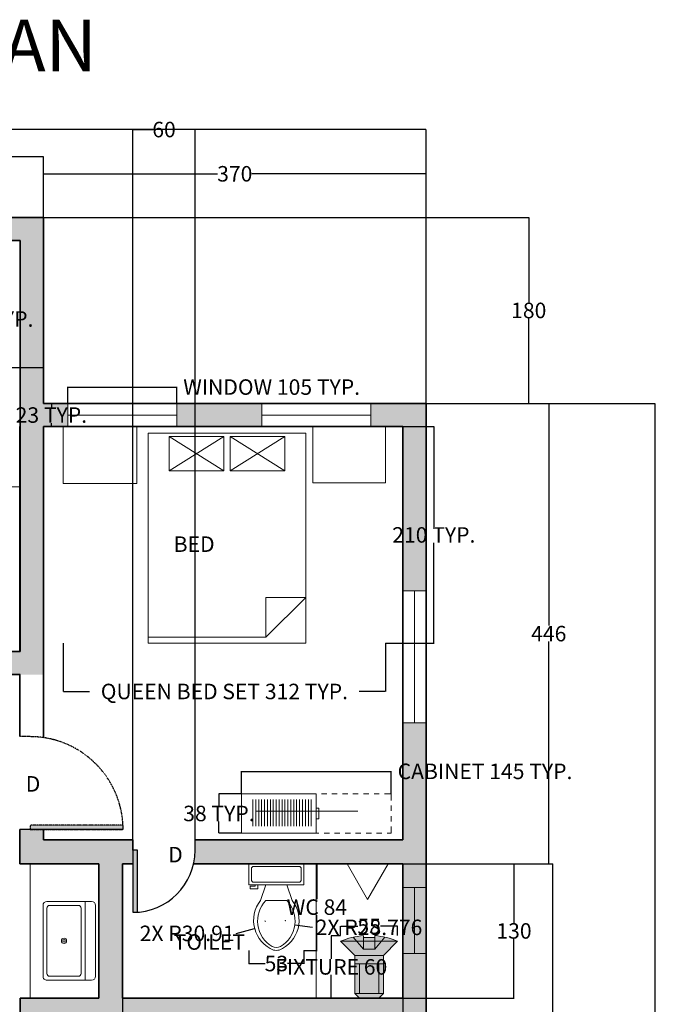
# Model space of a CAD drawing. Units: centimetres. Extents: x 355 to 1615, y 1030 to 2729.
# Tile 3 of 3: x 978 to 1615, y 1776 to 2729. Entities that reach past the tile are written whole.
import ezdxf

# ---------------------------------------------------------------- set-up
doc = ezdxf.new("R2010")
doc.units = ezdxf.units.CM
doc.header["$MEASUREMENT"] = 0
doc.linetypes.add('HIDDEN', pattern=[0.375, 0.25, -0.125])
for name, color, linetype, lineweight in [('A-ANNO-DIMS', 2, 'Continuous', 18), ('A-ANNO-TEXT', 7, 'Continuous', 25), ('A-AREA-IDEN', 7, 'Continuous', 25), ('A-DOOR', 4, 'Continuous', 25), ('A-DOOR-HIDN', 4, 'HIDDEN', 25), ('A-FLOR-CASE', 9, 'Continuous', 20), ('A-FLOR-FIXT', 9, 'Continuous', 18), ('A-FURN', 8, 'Continuous', 18), ('A-GLAZ', 4, 'Continuous', 18), ('A-WALL', 7, 'Continuous', 35), ('A-WALL-PATT', 5, 'Continuous', 13)]:
    doc.layers.add(name, color=color, linetype=linetype, lineweight=lineweight)
doc.styles.get("Standard").update_dxf_attribs({"font": 'arial.ttf'})
doc.dimstyles.get("Standard").update_dxf_attribs({"dimtxt": 15, "dimasz": 0.18, "dimexe": 0.18, "dimexo": 0.0625, "dimgap": 0.09, "dimtad": 0, "dimtih": 1, "dimtoh": 1, "dimdec": 0, "dimzin": 0, "dimdsep": 46, "dimtxsty": 'Standard', "dimcen": 0.09, "dimadec": 0, "dimazin": 0, "dimtfac": 1, "dimtdec": 0, "dimtofl": 0, "dimtmove": 0, "dimatfit": 3, "dimfxl": 1, "dimtolj": 1, "dimtzin": 0, "dimarcsym": 0})

# ---------------------------------------------------------------- blocks, each defined once
blk = doc.blocks.new('*D8')
at = {"layer": 'A-ANNO-DIMS', "color": 0, "lineweight": -2, "transparency": 16777216}
for p, q in [((611.23, 2537.61), (611.23, 2391.81)), ((1001.23, 2537.61), (1001.23, 2391.81)), ((611.41, 2391.99), (789.6, 2391.99)), ((1001.05, 2391.99), (822.86, 2391.99))]:
    blk.add_line(p, q, dxfattribs=at)
at = {"layer": 'A-ANNO-DIMS', "color": 0, "transparency": 16777216}
for points in [[(611.41, 2392.02), (611.41, 2391.96), (611.23, 2391.99)], [(1001.05, 2392.02), (1001.05, 2391.96), (1001.23, 2391.99)]]:
    blk.add_solid(points, dxfattribs=at)
at = {"layer": 'Defpoints', "color": 0, "transparency": 16777216}
for p in [(611.23, 2537.67), (1001.23, 2537.67), (1001.23, 2391.99)]:
    blk.add_point(p, dxfattribs=at)
at = {"layer": 'A-ANNO-DIMS', "color": 0, "transparency": 16777216, "insert": (806.23, 2391.99), "char_height": 15, "attachment_point": 5}
blk.add_mtext('\\A1;390', dxfattribs=at)
blk = doc.blocks.new('*U3')
for p, q in [((0, 0), (0, -100)), ((-900, 0), (-900, -100))]:
    blk.add_line(p, q)
blk.add_lwpolyline([(0, 0), (0, 900), (-43.75, 900), (-43.75, 0)], close=True)
blk.add_arc((0, 0), 900, 90, 180)
blk = doc.blocks.new('*U14')
for p, q in [((0, 0), (0, 100)), ((600, 0), (600, 100))]:
    blk.add_line(p, q)
blk.add_lwpolyline([(0, 0), (0, -600), (43.75, -600), (43.75, 0)], close=True)
blk.add_arc((0, 0), 600, 270, 0)
blk = doc.blocks.new('Toilet - top')
for p, q in [((9.5, -6), (9.5, -2)), ((-10, -8.5), (-8, -8.5)), ((-10, -9.5), (-10, -8.5)), ((-7, -9.5), (-10, -9.5)), ((-8, -8.5), (-8, -8)), ((-7, -8), (-7, -9.5)), ((-4, -8), (-6, -14)), ((4, -8), (6, -14)), ((4, -14), (-4, -14))]:
    blk.add_line(p, q)
blk.add_lwpolyline([(10.5, -8), (10.5, 0), (-10.5, 0), (-10.5, -8)], close=True)
for points in [[(-9.5, -2), (-9.5, -6)], [(8.5, -1), (-8.5, -1)], [(-8.5, -7), (8.5, -7)]]:
    blk.add_lwpolyline(points)
for centre, radius, start, end in [((-8.62, -1.88), 0.884, 81.8699, 188.1301), ((8.62, -1.88), 0.884, 351.8699, 98.1301), ((-8.62, -6.12), 0.884, 171.8699, 278.1301), ((8.62, -6.12), 0.884, 261.8699, 8.1301), ((3.52, -21.58), 12.17, 141.4691, 247.9714), ((4.2, -21.82), 11.33, 136.3677, 238.9468), ((-3.52, -21.58), 12.17, 292.0284, 38.5307), ((-4.2, -21.82), 11.33, 301.053, 43.6321), ((0, -27.88), 4, 245.7318, 294.2682), ((0, -29), 4, 254.8605, 285.1395)]:
    blk.add_arc(centre, radius, start, end)
blk = doc.blocks.new('Sink-single - 30 in top')
blk.add_line((-15, -3.999996), (15, -3.999996))
for points in [[(-13.5, 0), (13.5, 0)], [(-15, -18.499996), (-15, -1.5)], [(15, -1.5), (15, -18.499996)], [(-13.5, -17.499996), (-13.5, -6.499996)], [(-12.5, -5.499996), (12.5, -5.499996)], [(13.5, -6.499996), (13.5, -17.499996)], [(12.5, -18.499996), (-12.5, -18.499996)], [(13.5, -19.999996), (-13.5, -19.999996)]]:
    blk.add_lwpolyline(points)
for radius in [1, 0.5]:
    blk.add_circle((0, -11.999996), radius)
for centre, radius, start, end in [((-13.5, -1.5), 1.5, 90, 180), ((13.5, -1.5), 1.5, 0, 90), ((-12.5, -6.499996), 1, 90, 180), ((12.5, -6.499996), 1, 0, 90), ((-13.5, -18.499996), 1.5, 180, 270), ((-12.5, -17.499996), 1, 180, 270), ((12.5, -17.499996), 1, 270, 0), ((13.5, -18.499996), 1.5, 270, 0)]:
    blk.add_arc(centre, radius, start, end)
blk = doc.blocks.new('Cross Pt Oval Head Screw - 10 x 20 mm side')
at = {"color": 0}
for p, q in [((0.69, 12.04), (0.69, -7.65)), ((0.69, 12.04), (5.61, 7.12)), ((3.5, 4.16), (-0.69, 7.65)), ((18.75, 7.12), (5.61, 7.12)), ((5.61, 7.12), (5.61, -2.73)), ((8.56, -2.73), (8.56, 7.12)), ((18.75, -2.73), (18.75, 7.12)), ((20.38, 5.49), (18.75, 7.12)), ((-1.2, 4.16), (-0.61, 4.16)), ((3.5, 4.16), (-0.69, 4.16)), ((-0.61, 4.16), (-0.61, 0.23)), ((3.5, 4.16), (3.5, 0.23)), ((18.75, 5.49), (8.56, 5.49)), ((20.38, -1.1), (20.38, 5.49)), ((-1.2, 0.23), (-0.61, 0.23)), ((3.5, 0.23), (-0.69, 0.23)), ((3.5, 0.23), (-0.69, -3.26)), ((0.69, -7.65), (5.61, -2.73)), ((18.75, -2.73), (5.61, -2.73)), ((18.75, -1.1), (8.56, -1.1)), ((20.38, -1.1), (18.75, -2.73))]:
    blk.add_line(p, q, dxfattribs=at)
for start, end in [(157.3801, 175.5883), (184.4117, 202.6199)]:
    blk.add_arc((24.31, 2.19), 25.59, start, end, dxfattribs=at)
blk = doc.blocks.new('*D24')
at = {"layer": 'A-ANNO-DIMS', "color": 0, "lineweight": -2, "transparency": 16777216}
for p, q in [((611.23, 2537.73), (611.23, 2596.51)), ((611.41, 2596.33), (789.6, 2596.33)), ((1001.05, 2596.33), (822.86, 2596.33)), ((1001.23, 2537.73), (1001.23, 2596.51))]:
    blk.add_line(p, q, dxfattribs=at)
at = {"layer": 'A-ANNO-DIMS', "color": 0, "transparency": 16777216}
for points in [[(611.41, 2596.36), (611.41, 2596.3), (611.23, 2596.33)], [(1001.05, 2596.36), (1001.05, 2596.3), (1001.23, 2596.33)]]:
    blk.add_solid(points, dxfattribs=at)
at = {"layer": 'Defpoints', "color": 0, "transparency": 16777216}
for p in [(1001.23, 2596.33), (611.23, 2537.67), (1001.23, 2537.67)]:
    blk.add_point(p, dxfattribs=at)
at = {"layer": 'A-ANNO-DIMS', "color": 0, "transparency": 16777216, "insert": (806.23, 2596.33), "char_height": 15, "attachment_point": 5}
blk.add_mtext('\\A1;390', dxfattribs=at)
blk = doc.blocks.new('*D25')
at = {"layer": 'A-ANNO-DIMS', "color": 0, "lineweight": -2, "transparency": 16777216}
for p, q in [((1001.23, 2357.73), (1001.23, 2580.06)), ((1001.41, 2579.88), (1169.6, 2579.88)), ((1371.05, 2579.88), (1202.86, 2579.88)), ((1371.23, 2357.73), (1371.23, 2580.06))]:
    blk.add_line(p, q, dxfattribs=at)
at = {"layer": 'A-ANNO-DIMS', "color": 0, "transparency": 16777216}
for points in [[(1001.41, 2579.91), (1001.41, 2579.85), (1001.23, 2579.88)], [(1371.05, 2579.91), (1371.05, 2579.85), (1371.23, 2579.88)]]:
    blk.add_solid(points, dxfattribs=at)
at = {"layer": 'Defpoints', "color": 0, "transparency": 16777216}
for p in [(1371.23, 2579.88), (1001.23, 2357.67), (1371.23, 2357.67)]:
    blk.add_point(p, dxfattribs=at)
at = {"layer": 'A-ANNO-DIMS', "color": 0, "transparency": 16777216, "insert": (1186.23, 2579.88), "char_height": 15, "attachment_point": 5}
blk.add_mtext('\\A1;370', dxfattribs=at)
blk = doc.blocks.new('*D26')
at = {"layer": 'A-ANNO-DIMS', "color": 0, "lineweight": -2, "transparency": 16777216}
for p, q in [((1001.29, 2537.67), (1470.72, 2537.67)), ((1470.54, 2537.49), (1470.54, 2455.42)), ((1470.54, 2357.85), (1470.54, 2439.92)), ((1001.29, 2357.67), (1470.72, 2357.67))]:
    blk.add_line(p, q, dxfattribs=at)
at = {"layer": 'A-ANNO-DIMS', "color": 0, "transparency": 16777216}
for points in [[(1470.51, 2537.49), (1470.57, 2537.49), (1470.54, 2537.67)], [(1470.51, 2357.85), (1470.57, 2357.85), (1470.54, 2357.67)]]:
    blk.add_solid(points, dxfattribs=at)
at = {"layer": 'Defpoints', "color": 0, "transparency": 16777216}
for p in [(1001.23, 2537.67), (1001.23, 2357.67), (1470.54, 2357.67)]:
    blk.add_point(p, dxfattribs=at)
at = {"layer": 'A-ANNO-DIMS', "color": 0, "transparency": 16777216, "insert": (1470.54, 2447.67), "char_height": 15, "attachment_point": 5}
blk.add_mtext('\\A1;180', dxfattribs=at)
blk = doc.blocks.new('*D27')
at = {"layer": 'A-ANNO-DIMS', "color": 0, "lineweight": -2, "transparency": 16777216}
for p, q in [((1371.29, 2357.67), (1490.09, 2357.67)), ((1489.91, 2357.49), (1489.91, 2142.67)), ((1489.91, 1912.35), (1489.91, 2127.17)), ((1371.29, 1912.17), (1490.09, 1912.17))]:
    blk.add_line(p, q, dxfattribs=at)
at = {"layer": 'A-ANNO-DIMS', "color": 0, "transparency": 16777216}
for points in [[(1489.88, 2357.49), (1489.94, 2357.49), (1489.91, 2357.67)], [(1489.88, 1912.35), (1489.94, 1912.35), (1489.91, 1912.17)]]:
    blk.add_solid(points, dxfattribs=at)
at = {"layer": 'Defpoints', "color": 0, "transparency": 16777216}
for p in [(1371.23, 2357.67), (1371.23, 1912.17), (1489.91, 1912.17)]:
    blk.add_point(p, dxfattribs=at)
at = {"layer": 'A-ANNO-DIMS', "color": 0, "transparency": 16777216, "insert": (1489.91, 2134.92), "char_height": 15, "attachment_point": 5}
blk.add_mtext('\\A1;446', dxfattribs=at)
blk = doc.blocks.new('*D28')
at = {"layer": 'A-ANNO-DIMS', "color": 0, "lineweight": -2, "transparency": 16777216}
for p, q in [((1371.29, 1912.17), (1493.69, 1912.17)), ((1493.51, 1911.99), (1493.51, 1531.34)), ((1493.51, 1135.51), (1493.51, 1516.16)), ((1371.29, 1135.33), (1493.69, 1135.33))]:
    blk.add_line(p, q, dxfattribs=at)
at = {"layer": 'A-ANNO-DIMS', "color": 0, "transparency": 16777216}
for points in [[(1493.48, 1911.99), (1493.54, 1911.99), (1493.51, 1912.17)], [(1493.48, 1135.51), (1493.54, 1135.51), (1493.51, 1135.33)]]:
    blk.add_solid(points, dxfattribs=at)
at = {"layer": 'Defpoints', "color": 0, "transparency": 16777216}
for p in [(1371.23, 1912.17), (1371.23, 1135.33), (1493.51, 1135.33)]:
    blk.add_point(p, dxfattribs=at)
at = {"layer": 'A-ANNO-DIMS', "color": 0, "transparency": 16777216, "insert": (1493.51, 1523.75), "char_height": 15, "attachment_point": 5}
blk.add_mtext('\\A1;777', dxfattribs=at)
blk = doc.blocks.new('*D29')
at = {"layer": 'A-ANNO-DIMS', "color": 0, "lineweight": -2, "transparency": 16777216}
for p, q in [((1371.29, 2357.67), (1592.65, 2357.67)), ((1592.47, 2357.49), (1592.47, 1754.12)), ((1592.47, 1135.51), (1592.47, 1738.88)), ((1371.29, 1135.33), (1592.65, 1135.33))]:
    blk.add_line(p, q, dxfattribs=at)
at = {"layer": 'A-ANNO-DIMS', "color": 0, "transparency": 16777216}
for points in [[(1592.44, 2357.49), (1592.5, 2357.49), (1592.47, 2357.67)], [(1592.44, 1135.51), (1592.5, 1135.51), (1592.47, 1135.33)]]:
    blk.add_solid(points, dxfattribs=at)
at = {"layer": 'Defpoints', "color": 0, "transparency": 16777216}
for p in [(1371.23, 2357.67), (1371.23, 1135.33), (1592.47, 1135.33)]:
    blk.add_point(p, dxfattribs=at)
at = {"layer": 'A-ANNO-DIMS', "color": 0, "transparency": 16777216, "insert": (1592.47, 1746.5), "char_height": 15, "attachment_point": 5}
blk.add_mtext('\\A1;1222', dxfattribs=at)
blk = doc.blocks.new('BED-QUEEN-WITH-NIGHTSTANDS')
for p, q in [((82.24, 0), (82.24, 203.2)), ((82.24, 203.2), (234.64, 203.2)), ((102.56, 200.15), (155.39, 200.15)), ((102.56, 166.62), (102.56, 200.15)), ((102.56, 200.15), (155.39, 166.62)), ((102.56, 166.62), (155.39, 200.15)), ((155.39, 200.15), (155.39, 166.62)), ((161.48, 200.15), (214.32, 200.15)), ((161.48, 166.62), (161.48, 200.15)), ((161.48, 200.15), (214.32, 166.62)), ((161.48, 166.62), (214.32, 200.15)), ((214.32, 200.15), (214.32, 166.62)), ((234.64, 203.2), (234.64, 0)), ((155.39, 166.62), (102.56, 166.62)), ((161.48, 166.62), (214.32, 166.62)), ((234.64, 44.34), (196.03, 5.73)), ((196.03, 44.34), (234.64, 44.34)), ((196.03, 5.73), (196.03, 44.34)), ((82.24, 5.73), (196.03, 5.73)), ((234.64, 0), (82.24, 0))]:
    blk.add_line(p, q)
for points in [[(71.16, 209.52), (0, 209.52), (0, 154.37), (71.16, 154.37)], [(241.27, 209.52), (311.65, 209.52), (311.65, 155.31), (241.27, 155.31)]]:
    blk.add_lwpolyline(points, close=True)
blk = doc.blocks.new('File Cabinet - Letter')
for p, q in [((0, 0), (15, 0)), ((0, -28.5), (0, 0)), ((15, 0), (15, -28.5)), ((15, -28.5), (0, -28.5)), ((0, -29.5), (0, -28.5)), ((5.5, -28.5), (5.5, -29.5)), ((5.5, -29.5), (9.5, -29.5)), ((9.5, -29.5), (9.5, -28.5)), ((0, -33.5), (0, -31.5)), ((15, -30.5), (15, -32.5)), ((0, -37.5), (0, -35.5)), ((15, -34.5), (15, -36.5)), ((0, -41.5), (0, -39.5)), ((15, -38.5), (15, -40.5)), ((0, -45.5), (0, -43.5)), ((15, -42.5), (15, -44.5)), ((0, -49.5), (0, -47.5)), ((15, -46.5), (15, -48.5)), ((0, -53.5), (0, -51.5)), ((15, -50.5), (15, -52.5)), ((0, -57), (0, -55.5)), ((15, -54.5), (15, -57)), ((2.5, -57), (0, -57)), ((6.5, -57), (4.5, -57)), ((10.5, -57), (8.5, -57)), ((15, -57), (12.5, -57))]:
    blk.add_line(p, q)
blk = doc.blocks.new('BEDROOM-STORAGE-CABINET')
for p, q in [((11.1, 32.57), (11.1, 6.71)), ((13.92, 32.57), (13.92, 6.71)), ((16.74, 32.57), (16.74, 6.71)), ((19.57, 32.57), (19.57, 6.71)), ((22.39, 32.57), (22.39, 6.71)), ((25.22, 32.57), (25.22, 6.71)), ((28.04, 32.57), (28.04, 6.71)), ((30.87, 32.57), (30.87, 6.71)), ((33.69, 32.57), (33.69, 6.71)), ((36.51, 32.57), (36.51, 6.71)), ((39.34, 32.57), (39.34, 6.71)), ((42.16, 32.57), (42.16, 6.71)), ((44.99, 32.57), (44.99, 6.71)), ((47.81, 32.57), (47.81, 6.71)), ((50.64, 32.57), (50.64, 6.71)), ((53.46, 32.57), (53.46, 6.71)), ((56.29, 32.57), (56.29, 6.71)), ((59.11, 32.57), (59.11, 6.71)), ((61.93, 32.57), (61.93, 6.71)), ((64.76, 32.57), (64.76, 6.71)), ((67.58, 32.57), (67.58, 6.71)), ((13.92, 21.29), (112.77, 21.29))]:
    blk.add_line(p, q)
at = {"xscale": 2.54, "yscale": 2.54, "zscale": 2.54, "rotation": 90}
blk.add_blockref('File Cabinet - Letter', (0, 0), dxfattribs=at)
blk = doc.blocks.new('WIN-1054')
blk.add_line((0, 11.25), (105.44, 11.25))
blk.add_lwpolyline([(0, 22.5), (105.44, 22.5), (105.44, 0), (0, 0)], close=True)
blk = doc.blocks.new('WIN-640')
blk.add_line((11.25, 64.05), (11.25, 0))
blk.add_lwpolyline([(0, 64.05), (22.5, 64.05), (22.5, 0), (0, 0)], close=True)
blk = doc.blocks.new('*D38')
at = {"layer": 'A-ANNO-DIMS', "color": 0, "lineweight": -2, "transparency": 16777216}
for p, q in [((1024.66, 2357.73), (1024.66, 2373.67)), ((1024.84, 2373.49), (1129.92, 2373.49)), ((1130.1, 2357.73), (1130.1, 2373.67)), ((1130.1, 2373.49), (1130.28, 2373.49))]:
    blk.add_line(p, q, dxfattribs=at)
at = {"layer": 'A-ANNO-DIMS', "color": 0, "transparency": 16777216}
for points in [[(1024.84, 2373.52), (1024.84, 2373.46), (1024.66, 2373.49)], [(1129.92, 2373.52), (1129.92, 2373.46), (1130.1, 2373.49)]]:
    blk.add_solid(points, dxfattribs=at)
at = {"layer": 'Defpoints', "color": 0, "transparency": 16777216}
for p in [(1130.1, 2373.49), (1024.66, 2357.67), (1130.1, 2357.67)]:
    blk.add_point(p, dxfattribs=at)
at = {"layer": 'A-ANNO-DIMS', "color": 0, "transparency": 16777216, "insert": (1221.9, 2373.49), "char_height": 15, "attachment_point": 5}
blk.add_mtext('\\A1;WINDOW 105 TYP.', dxfattribs=at)
blk = doc.blocks.new('*D39')
at = {"layer": 'A-ANNO-DIMS', "color": 0, "lineweight": -2, "transparency": 16777216}
for p, q in [((1024.6, 2357.67), (1008.67, 2357.67)), ((1008.85, 2357.49), (1008.85, 2354.17)), ((1024.6, 2335.17), (1008.67, 2335.17)), ((1008.85, 2335.35), (1008.85, 2338.67))]:
    blk.add_line(p, q, dxfattribs=at)
at = {"layer": 'A-ANNO-DIMS', "color": 0, "transparency": 16777216}
for points in [[(1008.82, 2357.49), (1008.88, 2357.49), (1008.85, 2357.67)], [(1008.82, 2335.35), (1008.88, 2335.35), (1008.85, 2335.17)]]:
    blk.add_solid(points, dxfattribs=at)
at = {"layer": 'Defpoints', "color": 0, "transparency": 16777216}
for p in [(1008.85, 2357.67), (1024.66, 2357.67), (1024.66, 2335.17)]:
    blk.add_point(p, dxfattribs=at)
at = {"layer": 'A-ANNO-DIMS', "color": 0, "transparency": 16777216, "insert": (1008.85, 2346.42), "char_height": 15, "attachment_point": 5}
blk.add_mtext('\\A1;23 TYP.', dxfattribs=at)
blk = doc.blocks.new('*D44')
at = {"layer": 'A-ANNO-DIMS', "color": 0, "lineweight": -2, "transparency": 16777216}
for p, q in [((791.29, 2450.77), (791.29, 2439.22)), ((867.49, 2450.77), (867.49, 2439.22)), ((791.47, 2439.4), (867.31, 2439.4)), ((867.49, 2439.4), (867.67, 2439.4))]:
    blk.add_line(p, q, dxfattribs=at)
at = {"layer": 'A-ANNO-DIMS', "color": 0, "transparency": 16777216}
for points in [[(791.47, 2439.43), (791.47, 2439.37), (791.29, 2439.4)], [(867.31, 2439.43), (867.31, 2439.37), (867.49, 2439.4)]]:
    blk.add_solid(points, dxfattribs=at)
at = {"layer": 'Defpoints', "color": 0, "transparency": 16777216}
for p in [(791.29, 2450.83), (867.49, 2450.83), (867.49, 2439.4)]:
    blk.add_point(p, dxfattribs=at)
at = {"layer": 'A-ANNO-DIMS', "color": 0, "transparency": 16777216, "insert": (931.59, 2439.4), "char_height": 15, "attachment_point": 5}
blk.add_mtext('\\A1;SINK 76 TYP.', dxfattribs=at)
blk = doc.blocks.new('*D46')
at = {"layer": 'A-ANNO-DIMS', "color": 0, "lineweight": -2, "transparency": 16777216}
for p, q in [((1020.36, 2125.59), (1020.36, 2078.72)), ((1332.01, 2125.59), (1332.01, 2078.72)), ((1020.54, 2078.9), (1045.86, 2078.9)), ((1331.83, 2078.9), (1306.51, 2078.9))]:
    blk.add_line(p, q, dxfattribs=at)
at = {"layer": 'A-ANNO-DIMS', "color": 0, "transparency": 16777216}
for points in [[(1020.54, 2078.93), (1020.54, 2078.87), (1020.36, 2078.9)], [(1331.83, 2078.93), (1331.83, 2078.87), (1332.01, 2078.9)]]:
    blk.add_solid(points, dxfattribs=at)
at = {"layer": 'Defpoints', "color": 0, "transparency": 16777216}
for p in [(1020.36, 2125.65), (1332.01, 2125.65), (1332.01, 2078.9)]:
    blk.add_point(p, dxfattribs=at)
at = {"layer": 'A-ANNO-DIMS', "color": 0, "transparency": 16777216, "insert": (1176.19, 2078.9), "char_height": 15, "attachment_point": 5}
blk.add_mtext('\\A1;QUEEN BED SET 312 TYP.', dxfattribs=at)
blk = doc.blocks.new('*D47')
at = {"layer": 'A-ANNO-DIMS', "color": 0, "lineweight": -2, "transparency": 16777216}
for p, q in [((1332.07, 2335.17), (1378.94, 2335.17)), ((1378.76, 2334.99), (1378.76, 2238.16)), ((1378.76, 2125.83), (1378.76, 2222.66)), ((1332.07, 2125.65), (1378.94, 2125.65))]:
    blk.add_line(p, q, dxfattribs=at)
at = {"layer": 'A-ANNO-DIMS', "color": 0, "transparency": 16777216}
for points in [[(1378.73, 2334.99), (1378.79, 2334.99), (1378.76, 2335.17)], [(1378.73, 2125.83), (1378.79, 2125.83), (1378.76, 2125.65)]]:
    blk.add_solid(points, dxfattribs=at)
at = {"layer": 'Defpoints', "color": 0, "transparency": 16777216}
for p in [(1332.01, 2335.17), (1378.76, 2335.17), (1332.01, 2125.65)]:
    blk.add_point(p, dxfattribs=at)
at = {"layer": 'A-ANNO-DIMS', "color": 0, "transparency": 16777216, "insert": (1378.76, 2230.41), "char_height": 15, "attachment_point": 5}
blk.add_mtext('\\A1;210 TYP.', dxfattribs=at)
blk = doc.blocks.new('*D48')
at = {"layer": 'A-ANNO-DIMS', "color": 0, "lineweight": -2, "transparency": 16777216}
for p, q in [((1192.63, 1979.94), (1192.63, 2001.77)), ((1192.81, 2001.59), (1337.23, 2001.59)), ((1337.41, 1979.94), (1337.41, 2001.77)), ((1337.41, 2001.59), (1337.59, 2001.59))]:
    blk.add_line(p, q, dxfattribs=at)
at = {"layer": 'A-ANNO-DIMS', "color": 0, "transparency": 16777216}
for points in [[(1192.81, 2001.62), (1192.81, 2001.56), (1192.63, 2001.59)], [(1337.23, 2001.62), (1337.23, 2001.56), (1337.41, 2001.59)]]:
    blk.add_solid(points, dxfattribs=at)
at = {"layer": 'Defpoints', "color": 0, "transparency": 16777216}
for p in [(1337.41, 2001.59), (1192.63, 1979.88), (1337.41, 1979.88)]:
    blk.add_point(p, dxfattribs=at)
at = {"layer": 'A-ANNO-DIMS', "color": 0, "transparency": 16777216, "insert": (1428.25, 2001.59), "char_height": 15, "attachment_point": 5}
blk.add_mtext('\\A1;CABINET 145 TYP.', dxfattribs=at)
blk = doc.blocks.new('*D49')
at = {"layer": 'A-ANNO-DIMS', "color": 0, "lineweight": -2, "transparency": 16777216}
for p, q in [((1192.57, 1979.88), (1170.73, 1979.88)), ((1170.91, 1979.7), (1170.91, 1968.58)), ((1170.91, 1941.96), (1170.91, 1953.07)), ((1192.57, 1941.78), (1170.73, 1941.78))]:
    blk.add_line(p, q, dxfattribs=at)
at = {"layer": 'A-ANNO-DIMS', "color": 0, "transparency": 16777216}
for points in [[(1170.88, 1979.7), (1170.94, 1979.7), (1170.91, 1979.88)], [(1170.88, 1941.96), (1170.94, 1941.96), (1170.91, 1941.78)]]:
    blk.add_solid(points, dxfattribs=at)
at = {"layer": 'Defpoints', "color": 0, "transparency": 16777216}
for p in [(1170.91, 1979.88), (1192.63, 1979.88), (1192.63, 1941.78)]:
    blk.add_point(p, dxfattribs=at)
at = {"layer": 'A-ANNO-DIMS', "color": 0, "transparency": 16777216, "insert": (1170.91, 1960.83), "char_height": 15, "attachment_point": 5}
blk.add_mtext('\\A1;38 TYP.', dxfattribs=at)
blk = doc.blocks.new('*D54')
at = {"layer": 'A-ANNO-DIMS', "color": 0, "lineweight": -2, "transparency": 16777216}
for p, q in [((1253.17, 1912.17), (1265.88, 1912.17)), ((1265.7, 1911.99), (1265.7, 1878.05)), ((1265.7, 1828.41), (1265.7, 1862.36)), ((1253.17, 1828.23), (1265.88, 1828.23))]:
    blk.add_line(p, q, dxfattribs=at)
at = {"layer": 'A-ANNO-DIMS', "color": 0, "transparency": 16777216}
for points in [[(1265.67, 1911.99), (1265.73, 1911.99), (1265.7, 1912.17)], [(1265.67, 1828.41), (1265.73, 1828.41), (1265.7, 1828.23)]]:
    blk.add_solid(points, dxfattribs=at)
at = {"layer": 'Defpoints', "color": 0, "transparency": 16777216}
for p in [(1253.11, 1912.17), (1265.7, 1912.17), (1253.11, 1828.23)]:
    blk.add_point(p, dxfattribs=at)
at = {"layer": 'A-ANNO-DIMS', "color": 0, "transparency": 16777216, "insert": (1265.7, 1870.2), "char_height": 15, "attachment_point": 5}
blk.add_mtext('\\A1;WC 84', dxfattribs=at)
blk = doc.blocks.new('*D55')
at = {"layer": 'A-ANNO-DIMS', "color": 0, "lineweight": -2, "transparency": 16777216}
for p, q in [((1199.77, 1828.17), (1199.77, 1815.46)), ((1253.11, 1828.17), (1253.11, 1815.46)), ((1199.95, 1815.64), (1215.61, 1815.64)), ((1252.93, 1815.64), (1237.27, 1815.64))]:
    blk.add_line(p, q, dxfattribs=at)
at = {"layer": 'A-ANNO-DIMS', "color": 0, "transparency": 16777216}
for points in [[(1199.95, 1815.67), (1199.95, 1815.61), (1199.77, 1815.64)], [(1252.93, 1815.67), (1252.93, 1815.61), (1253.11, 1815.64)]]:
    blk.add_solid(points, dxfattribs=at)
at = {"layer": 'Defpoints', "color": 0, "transparency": 16777216}
for p in [(1199.77, 1828.23), (1253.11, 1828.23), (1253.11, 1815.64)]:
    blk.add_point(p, dxfattribs=at)
at = {"layer": 'A-ANNO-DIMS', "color": 0, "transparency": 16777216, "insert": (1226.44, 1815.64), "char_height": 15, "attachment_point": 5}
blk.add_mtext('\\A1;53', dxfattribs=at)
blk = doc.blocks.new('*D56')
at = {"layer": 'A-ANNO-DIMS', "color": 0, "lineweight": -2, "transparency": 16777216}
for p, q in [((1288.55, 1842.58), (1279.37, 1842.58)), ((1279.55, 1842.4), (1279.55, 1820.11)), ((1279.55, 1782.32), (1279.55, 1804.61)), ((1288.55, 1782.14), (1279.37, 1782.14))]:
    blk.add_line(p, q, dxfattribs=at)
at = {"layer": 'A-ANNO-DIMS', "color": 0, "transparency": 16777216}
for points in [[(1279.52, 1842.4), (1279.58, 1842.4), (1279.55, 1842.58)], [(1279.52, 1782.32), (1279.58, 1782.32), (1279.55, 1782.14)]]:
    blk.add_solid(points, dxfattribs=at)
at = {"layer": 'Defpoints', "color": 0, "transparency": 16777216}
for p in [(1288.61, 1842.58), (1279.55, 1782.14), (1288.61, 1782.14)]:
    blk.add_point(p, dxfattribs=at)
at = {"layer": 'A-ANNO-DIMS', "color": 0, "transparency": 16777216, "insert": (1279.55, 1812.36), "char_height": 15, "attachment_point": 5}
blk.add_mtext('\\A1;FIXTURE 60', dxfattribs=at)
blk = doc.blocks.new('*D57')
at = {"layer": 'A-ANNO-DIMS', "color": 0, "lineweight": -2, "transparency": 16777216}
for p, q in [((1288.61, 1842.64), (1288.61, 1851.83)), ((1288.79, 1851.65), (1305.29, 1851.65)), ((1343.57, 1851.65), (1327.07, 1851.65)), ((1343.75, 1842.64), (1343.75, 1851.83))]:
    blk.add_line(p, q, dxfattribs=at)
at = {"layer": 'A-ANNO-DIMS', "color": 0, "transparency": 16777216}
for points in [[(1288.79, 1851.68), (1288.79, 1851.62), (1288.61, 1851.65)], [(1343.57, 1851.68), (1343.57, 1851.62), (1343.75, 1851.65)]]:
    blk.add_solid(points, dxfattribs=at)
at = {"layer": 'Defpoints', "color": 0, "transparency": 16777216}
for p in [(1288.61, 1851.65), (1288.61, 1842.58), (1343.75, 1842.58)]:
    blk.add_point(p, dxfattribs=at)
at = {"layer": 'A-ANNO-DIMS', "color": 0, "transparency": 16777216, "insert": (1316.18, 1851.65), "char_height": 15, "attachment_point": 5}
blk.add_mtext('\\A1;55', dxfattribs=at)
blk = doc.blocks.new('*D64')
at = {"layer": 'A-ANNO-DIMS', "color": 0, "lineweight": -2, "transparency": 16777216}
for p, q in [((471.23, 2060.23), (471.23, 2622.9)), ((471.41, 2622.72), (904.6, 2622.72)), ((1371.05, 2622.72), (937.87, 2622.72)), ((1371.23, 2357.73), (1371.23, 2622.9))]:
    blk.add_line(p, q, dxfattribs=at)
at = {"layer": 'A-ANNO-DIMS', "color": 0, "transparency": 16777216}
for points in [[(471.41, 2622.75), (471.41, 2622.69), (471.23, 2622.72)], [(1371.05, 2622.75), (1371.05, 2622.69), (1371.23, 2622.72)]]:
    blk.add_solid(points, dxfattribs=at)
at = {"layer": 'Defpoints', "color": 0, "transparency": 16777216}
for p in [(1371.23, 2622.72), (1371.23, 2357.67), (471.23, 2060.17)]:
    blk.add_point(p, dxfattribs=at)
at = {"layer": 'A-ANNO-DIMS', "color": 0, "transparency": 16777216, "insert": (921.23, 2622.72), "char_height": 15, "attachment_point": 5}
blk.add_mtext('\\A1;900', dxfattribs=at)
blk = doc.blocks.new('*D66')
at = {"layer": 'A-ANNO-DIMS', "color": 0, "lineweight": -2, "transparency": 16777216}
for p, q in [((1077.8, 1782.11), (1077.8, 1050.1)), ((1348.73, 1782.11), (1348.73, 1050.1)), ((1077.98, 1050.28), (1181.91, 1050.28)), ((1348.55, 1050.28), (1244.62, 1050.28))]:
    blk.add_line(p, q, dxfattribs=at)
at = {"layer": 'A-ANNO-DIMS', "color": 0, "transparency": 16777216}
for points in [[(1077.98, 1050.31), (1077.98, 1050.25), (1077.8, 1050.28)], [(1348.55, 1050.31), (1348.55, 1050.25), (1348.73, 1050.28)]]:
    blk.add_solid(points, dxfattribs=at)
at = {"layer": 'Defpoints', "color": 0, "transparency": 16777216}
for p in [(1077.8, 1782.17), (1348.73, 1782.17), (1348.73, 1050.28)]:
    blk.add_point(p, dxfattribs=at)
at = {"layer": 'A-ANNO-DIMS', "color": 0, "transparency": 16777216, "insert": (1213.27, 1050.28), "char_height": 15, "attachment_point": 5}
blk.add_mtext('\\A1;270.93', dxfattribs=at)
blk = doc.blocks.new('*D67')
at = {"layer": 'A-ANNO-DIMS', "color": 0, "lineweight": -2, "transparency": 16777216}
for p, q in [((1348.79, 1912.17), (1456.46, 1912.17)), ((1456.28, 1911.99), (1456.28, 1854.92)), ((1456.28, 1782.35), (1456.28, 1839.42)), ((1348.79, 1782.17), (1456.46, 1782.17))]:
    blk.add_line(p, q, dxfattribs=at)
at = {"layer": 'A-ANNO-DIMS', "color": 0, "transparency": 16777216}
for points in [[(1456.25, 1911.99), (1456.31, 1911.99), (1456.28, 1912.17)], [(1456.25, 1782.35), (1456.31, 1782.35), (1456.28, 1782.17)]]:
    blk.add_solid(points, dxfattribs=at)
at = {"layer": 'Defpoints', "color": 0, "transparency": 16777216}
for p in [(1348.73, 1912.17), (1456.28, 1912.17), (1348.73, 1782.17)]:
    blk.add_point(p, dxfattribs=at)
at = {"layer": 'A-ANNO-DIMS', "color": 0, "transparency": 16777216, "insert": (1456.28, 1847.17), "char_height": 15, "attachment_point": 5}
blk.add_mtext('\\A1;130', dxfattribs=at)
blk = doc.blocks.new('*D72')
at = {"layer": 'A-ANNO-DIMS', "color": 0, "lineweight": -2, "transparency": 16777216}
for p, q in [((1087.8, 1935.23), (1087.8, 2622.9)), ((1087.98, 2622.72), (1106.96, 2622.72)), ((1147.62, 2622.72), (1128.65, 2622.72)), ((1147.8, 1935.23), (1147.8, 2622.9))]:
    blk.add_line(p, q, dxfattribs=at)
at = {"layer": 'A-ANNO-DIMS', "color": 0, "transparency": 16777216}
for points in [[(1087.98, 2622.75), (1087.98, 2622.69), (1087.8, 2622.72)], [(1147.62, 2622.75), (1147.62, 2622.69), (1147.8, 2622.72)]]:
    blk.add_solid(points, dxfattribs=at)
at = {"layer": 'Defpoints', "color": 0, "transparency": 16777216}
for p in [(1147.8, 2622.72), (1087.8, 1935.17), (1147.8, 1935.17)]:
    blk.add_point(p, dxfattribs=at)
at = {"layer": 'A-ANNO-DIMS', "color": 0, "transparency": 16777216, "insert": (1117.8, 2622.72), "char_height": 15, "attachment_point": 5}
blk.add_mtext('\\A1;60', dxfattribs=at)
blk = doc.blocks.new('*D80')
at = {"layer": 'A-ANNO-DIMS', "color": 0, "lineweight": -2, "transparency": 16777216}
for p, q in [((1187.55, 1844.79), (1205.31, 1849.46)), ((1235.29, 1857.36), (1235.47, 1857.36)), ((1235.38, 1857.27), (1235.38, 1857.45))]:
    blk.add_line(p, q, dxfattribs=at)
at = {"layer": 'A-ANNO-DIMS', "color": 0, "transparency": 16777216}
blk.add_solid([(1205.3, 1849.49), (1205.32, 1849.43), (1205.49, 1849.5)], dxfattribs=at)
at = {"layer": 'Defpoints', "color": 0, "transparency": 16777216}
for p in [(1205.49, 1849.5), (1235.38, 1857.36)]:
    blk.add_point(p, dxfattribs=at)
at = {"layer": 'A-ANNO-DIMS', "color": 0, "transparency": 16777216, "insert": (1140.18, 1844.79), "char_height": 15, "attachment_point": 5}
blk.add_mtext('\\A1;2X R30.91', dxfattribs=at)
blk = doc.blocks.new('*D81')
at = {"layer": 'A-ANNO-DIMS', "color": 0, "lineweight": -2, "transparency": 16777216}
for p, q in [((1215.68, 1856.75), (1215.86, 1856.75)), ((1215.77, 1856.66), (1215.77, 1856.84)), ((1261.4, 1850.62), (1244.47, 1852.9))]:
    blk.add_line(p, q, dxfattribs=at)
at = {"layer": 'A-ANNO-DIMS', "color": 0, "transparency": 16777216}
blk.add_solid([(1244.47, 1852.93), (1244.47, 1852.87), (1244.29, 1852.92)], dxfattribs=at)
at = {"layer": 'Defpoints', "color": 0, "transparency": 16777216}
for p in [(1215.77, 1856.75), (1244.29, 1852.92)]:
    blk.add_point(p, dxfattribs=at)
at = {"layer": 'A-ANNO-DIMS', "color": 0, "transparency": 16777216, "insert": (1316.05, 1850.62), "char_height": 15, "attachment_point": 5}
blk.add_mtext('\\A1;2X R28.776', dxfattribs=at)

msp = doc.modelspace()

# ---------------------------------------------------------------- hatches: boundary and pattern name
at = {"layer": 'A-WALL-PATT'}
h = msp.add_hatch(color=256, dxfattribs=at)
h.dxf.hatch_style = 1
h.paths.add_polyline_path([(1001.2322, 2537.6708), (931.0729, 2537.6708), (931.0729, 2515.1708), (978.7322, 2515.1708), (978.7322, 2117.6708), (968.7322, 2117.6708), (968.7322, 2095.1708), (978.7322, 2095.1708), (1001.2322, 2095.1708), (1001.2322, 2335.1708), (1024.6627, 2335.1708), (1024.6627, 2357.6708), (1001.2322, 2357.6708)])
h.paths.add_polyline_path([(611.2322, 2537.6708), (611.2322, 2217.6708), (611.4122, 2217.6708), (621.2322, 2217.6708, -0.03484893), (633.7322, 2216.7985), (633.7322, 2515.1708), (736.2344, 2515.1708), (736.2344, 2537.6708)])
h = msp.add_hatch(color=256, dxfattribs=at)
h.dxf.hatch_style = 1
h.paths.add_polyline_path([(1212.284, 2335.1708), (1212.284, 2357.6708), (1130.1042, 2357.6708), (1130.1042, 2335.1708)])
h.paths.add_polyline_path([(1371.2322, 2357.6708), (1317.7255, 2357.6708), (1317.7255, 2335.1708), (1348.7322, 2335.1708), (1348.7322, 2176.2951), (1371.2322, 2176.2951)])
h = msp.add_hatch(color=256, dxfattribs=at)
h.dxf.hatch_style = 1
h.paths.add_polyline_path([(611.2322, 1747.6708), (611.2322, 1583.8272), (633.7322, 1583.8272), (633.7322, 1747.6708), (794.4619, 1747.6708), (794.4619, 1770.1708), (563.7322, 1770.1708), (563.7322, 1828.1708), (471.2322, 1828.1708), (471.2322, 1805.1708), (541.2322, 1805.1708), (541.2322, 1747.6708)])
h.paths.add_polyline_path([(1371.2322, 2048.5797), (1348.7322, 2048.5797), (1348.7322, 1935.1708), (1147.8044, 1935.1708), (1147.8044, 1925.1708, -0.054654), (1146.3791, 1912.1708), (1348.7322, 1912.1708), (1348.7322, 1889.2147), (1371.2322, 1889.2147)])
h.paths.add_polyline_path([(988.2322, 1945.1708), (988.2322, 1949.5458), (1078.2322, 1949.5458), (1078.2322, 1945.1708), (1001.2322, 1945.1708), (1001.2322, 1935.1708), (1087.8044, 1935.1708), (1087.8044, 1925.1708), (1092.1794, 1925.1708), (1092.1794, 1865.1708), (1087.8044, 1865.1708), (1087.8044, 1912.1708), (1077.8044, 1912.1708), (1077.8044, 1782.1708), (1306.9174, 1782.1708), (1302.395, 1786.6932), (1302.395, 1823.4958), (1288.6113, 1837.2795, -0.07961558), (1310.6652, 1842.5806), (1310.6652, 1840.9346), (1321.6922, 1840.9346), (1321.6922, 1841.147), (1321.6922, 1842.5806, -0.07961558), (1343.7462, 1837.2795), (1329.9624, 1823.4958), (1329.9624, 1786.6932), (1325.44, 1782.1708), (1348.7322, 1782.1708), (1348.7322, 1889.2147), (1371.2322, 1889.2147), (1371.2322, 1605.3038), (1348.7322, 1605.3038), (1348.7322, 1767.1708), (978.7322, 1767.1708), (978.7322, 1782.1708), (1054.8044, 1782.1708), (1054.8044, 1912.1708), (978.2322, 1912.1708), (978.2322, 1945.1708)])
h.paths.add_polyline_path([(1371.2322, 1605.3038), (1348.7322, 1605.3038), (1348.7322, 1541.3252), (1111.7322, 1541.3252), (1111.7322, 1531.3252, -0.04358087), (1110.5969, 1518.3252), (1348.7322, 1518.3252), (1348.7322, 1403.9189), (1371.2322, 1403.9189)])
h.paths.add_polyline_path([(1173.1703, 1158.3252), (1173.1703, 1135.3252), (1225.9516, 1135.3252), (1225.9516, 1158.3252)])
h.paths.add_polyline_path([(648.3142, 1244.6708), (648.3142, 1267.6708), (633.7322, 1267.6708), (633.7322, 1388.9888), (611.2322, 1388.9888), (611.2322, 1267.6708), (541.2322, 1267.6708), (541.2322, 1244.6708)])
h.paths.add_polyline_path([(633.7322, 2117.6708), (633.7322, 2127.6708), (621.2322, 2127.6708), (611.2322, 2127.6708), (611.2322, 2117.6708), (541.2322, 2117.6708), (541.2322, 2060.1708), (471.2322, 2060.1708), (471.2322, 2037.1708), (563.7322, 2037.1708), (563.7322, 2095.1708), (878.7322, 2095.1708), (878.7322, 2105.1708, -0.03484893), (879.6045, 2117.6708)])
h.paths.add_polyline_path([(843.1527, 1267.3404), (843.1527, 1244.8404), (648.3142, 1244.8404), (648.3142, 1244.6708), (858.7322, 1244.6708), (858.7322, 1254.6708), (863.1072, 1254.6708), (863.1072, 1329.6708), (858.7322, 1329.6708), (858.7322, 1267.6708), (648.3142, 1267.6708), (648.3142, 1267.3404)])
h.paths.add_polyline_path([(1067.7288, 1135.8252), (1067.7288, 1158.3252), (1026.7322, 1158.3252), (1026.7322, 1518.3252), (1036.7322, 1518.3252), (1036.7322, 1456.3252), (1041.1072, 1456.3252), (1041.1072, 1531.3252), (1036.7322, 1531.3252), (1036.7322, 1541.3252), (1003.7322, 1541.3252), (1003.7322, 1267.6708), (993.7322, 1267.6708), (993.7322, 1314.6708), (989.3572, 1314.6708), (989.3572, 1254.6708), (993.7322, 1254.6708), (993.7322, 1244.6708), (1003.7322, 1244.6708), (1003.7322, 1135.3252), (1173.1703, 1135.3252), (1173.1703, 1135.8252)])

# ---------------------------------------------------------------- linework, layer by layer
at = {"layer": 'A-DOOR'}
msp.add_line((1078.2322, 1945.1708), (978.2322, 1945.1708), dxfattribs=at)
at = {"layer": 'A-FLOR-CASE'}
for p, q in [((873.4996, 2277.0056), (978.7322, 2277.0056)), ((988.2634, 1912.1708), (988.2634, 1782.1708))]:
    msp.add_line(p, q, dxfattribs=at)
at = {"layer": 'A-FLOR-FIXT'}
msp.add_line((1265.0464, 1912.1708), (1265.0464, 1782.1708), dxfattribs=at)
msp.add_lwpolyline([(1314.7173, 1877.6708), (1294.7988, 1912.1708), (1334.6359, 1912.1708)], close=True, dxfattribs=at)
at = {"layer": 'A-GLAZ'}
msp.add_line((1359.9822, 2176.2584), (1359.9822, 2048.5797), dxfattribs=at)
msp.add_lwpolyline([(1348.7322, 2176.2584), (1371.2322, 2176.2584), (1371.2322, 2048.5797), (1348.7322, 2048.5797)], close=True, dxfattribs=at)
at = {"layer": 'A-WALL'}
for p, q in [((1001.2322, 2537.6708), (611.2322, 2537.6708)), ((1001.2322, 2357.6708), (1001.2322, 2537.6708)), ((978.7322, 2515.1708), (633.7322, 2515.1708)), ((978.7322, 2117.6708), (978.7322, 2515.1708)), ((1371.2322, 2357.6708), (1001.2322, 2357.6708)), ((1371.2322, 1135.3252), (1371.2322, 2357.6708)), ((978.2322, 2117.6708), (978.2322, 2335.1708)), ((1001.2322, 2095.1708), (1001.2322, 2335.1708)), ((1348.7322, 2335.1708), (1001.2322, 2335.1708)), ((1001.2322, 2335.1708), (1348.7322, 2335.1708)), ((1001.2322, 2034.2269), (1001.2322, 2335.1708)), ((1348.7322, 1935.1708), (1348.7322, 2335.1708)), ((978.7322, 2117.6708), (968.7322, 2117.6708)), ((978.7322, 2095.1708), (968.7322, 2095.1708)), ((978.2322, 2035.1708), (978.2322, 2095.1708)), ((978.2322, 1912.1708), (978.2322, 1945.1708)), ((1001.2322, 1935.1708), (1001.2322, 1945.1708)), ((1087.8044, 1935.1708), (1001.2322, 1935.1708)), ((1087.8044, 1925.1708), (1087.8044, 1935.1708)), ((1348.7322, 1935.1708), (1147.8044, 1935.1708)), ((1054.8044, 1912.1708), (978.2322, 1912.1708)), ((1054.8044, 1912.1708), (978.7322, 1912.1708)), ((1054.8044, 1912.1708), (1054.8044, 1782.1708)), ((1077.8044, 1912.1708), (1077.8044, 1782.1708)), ((1087.8044, 1912.1708), (1077.8044, 1912.1708)), ((1087.8044, 1912.1708), (1077.8044, 1912.1708)), ((1348.7322, 1912.1708), (1146.3791, 1912.1708)), ((1348.7322, 1912.1708), (1146.3791, 1912.1708)), ((1348.7322, 1782.1708), (1348.7322, 1912.1708)), ((1348.7322, 1782.1708), (1348.7322, 1912.1708)), ((978.7322, 1782.1708), (1054.8044, 1782.1708)), ((978.7322, 1782.1708), (978.7322, 1767.1708)), ((1077.8044, 1782.1708), (1348.7322, 1782.1708))]:
    msp.add_line(p, q, dxfattribs=at)

# ---------------------------------------------------------------- block references
at = {"layer": 'A-DOOR', "xscale": 0.1, "yscale": 0.1, "zscale": 0.1}
msp.add_blockref('*U14', (1087.8044, 1925.1708), dxfattribs=at)
at = {"layer": 'A-DOOR-HIDN', "xscale": 0.1, "yscale": 0.1, "zscale": 0.1, "rotation": 270}
msp.add_blockref('*U3', (988.2322, 1945.1708), dxfattribs=at)
at = {"layer": 'A-FLOR-FIXT', "xscale": 2.54, "yscale": 2.54, "zscale": 2.54}
msp.add_blockref('Toilet - top', (1226.4401, 1912.1708), dxfattribs=at)
at = {"layer": 'A-FLOR-FIXT'}
for name, p, xscale, yscale, zscale, rotation in [('Sink-single - 30 in top', (1051.5639, 1837.5873), 2.54, 2.54, 2.54, 270), ('Cross Pt Oval Head Screw - 10 x 20 mm side', (1322.3262, 1839.2132), -2.800858940871992, 2.800858940871992, 2.800858940871992, 90)]:
    msp.add_blockref(name, p, dxfattribs=dict(at, xscale=xscale, yscale=yscale, zscale=zscale, rotation=rotation))
at = {"layer": 'A-FURN'}
for name, p in [('BED-QUEEN-WITH-NIGHTSTANDS', (1020.363, 2125.649)), ('BEDROOM-STORAGE-CABINET', (1192.628, 1941.777))]:
    msp.add_blockref(name, p, dxfattribs=at)
at = {"layer": 'A-GLAZ'}
for name, p in [('WIN-1054', (1024.663, 2335.171)), ('WIN-1054', (1212.2843, 2335.171)), ('WIN-640', (1348.732, 1825.167))]:
    msp.add_blockref(name, p, dxfattribs=at)

# ---------------------------------------------------------------- texts
at = {"layer": 'A-ANNO-TEXT', "attachment_point": 1}
for s, width, insert, char_height in [('PLAN', 884.916338, (881.6359, 2729.0182), 50), ('D', 33.654124, (984.0783, 1996.9772), 15), ('D', 33.654124, (1121.8315, 1928.4818), 15)]:
    msp.add_mtext_dynamic_manual_height_columns(s, width=width, gutter_width=1, heights=[0], dxfattribs=dict(at, insert=insert, char_height=char_height))
at = {"layer": 'A-AREA-IDEN', "char_height": 15, "attachment_point": 1}
for s, insert in [('BED', (1127.1496, 2228.9598)), ('TOILET', (1127.1496, 1843.9251))]:
    msp.add_mtext_dynamic_manual_height_columns(s, width=89.241844, gutter_width=1, heights=[0], dxfattribs=dict(at, insert=insert))

# ---------------------------------------------------------------- dimensions: what is measured, and where the dimension line sits
at = {"layer": 'A-ANNO-DIMS'}
for base, p1, p2, override, picture, middle in [((1371.2322, 2622.7208), (471.2322, 2060.1708), (1371.2322, 2357.6708), {"dimdec": 0, "dimlfac": 1, "dimrnd": 0, "dimzin": 0, "dimdsep": 46, "dimlunit": 2}, '*D64', (921.2322, 2622.7208)), ((1147.8044, 2622.7208), (1087.8044, 1935.1708), (1147.8044, 1935.1708), {"dimdec": 0, "dimlfac": 1, "dimrnd": 0, "dimzin": 0, "dimdsep": 46, "dimlunit": 2}, '*D72', (1117.8044, 2622.7208)), ((1001.2322, 2596.3337), (611.2322, 2537.6708), (1001.2322, 2537.6708), {"dimclrd": 0, "dimclre": 0, "dimclrt": 0}, '*D24', (806.2322, 2596.3337)), ((1371.2322, 2579.8787), (1001.2322, 2357.6708), (1371.2322, 2357.6708), {"dimclrd": 0, "dimclre": 0, "dimclrt": 0}, '*D25', (1186.2322, 2579.8787)), ((1001.2322, 2391.9927), (611.2322, 2537.6708), (1001.2322, 2537.6708), {"dimclrd": 0, "dimclre": 0, "dimclrt": 0}, '*D8', (806.2322, 2391.9927)), ((1253.1101, 1815.6427), (1199.7701, 1828.2333), (1253.1101, 1828.2333), {"dimdec": 0, "dimlfac": 1, "dimrnd": 0, "dimzin": 0, "dimdsep": 46, "dimlunit": 2}, '*D55', (1226.4401, 1815.6427)), ((1348.7322, 1050.2752), (1077.8044, 1782.1708), (1348.7322, 1782.1708), {"dimdec": 2, "dimlfac": 1, "dimrnd": 0, "dimzin": 0, "dimdsep": 46, "dimlunit": 2}, '*D66', (1213.2683, 1050.2752))]:
    dim = msp.add_linear_dim(base=base, p1=p1, p2=p2, dimstyle='Standard', override=override, dxfattribs=at)
    dim.commit()
    dim.dimension.update_dxf_attribs({"geometry": picture, "text_midpoint": middle})
for base, p1, p2, angle, override, picture, middle in [((1470.5426, 2357.6708), (1001.2322, 2537.6708), (1001.2322, 2357.6708), 90, {"dimclrd": 0, "dimclre": 0, "dimclrt": 0}, '*D26', (1470.5426, 2447.6708)), ((1489.9052441184, 1912.1707694651), (1371.2322031806, 2357.6707694651), (1371.2322031806, 1912.1707694651), 90, {"dimclrd": 0, "dimclre": 0, "dimclrt": 0}, '*D27', (1489.9052441184, 2134.9207694651)), ((1592.4723, 1135.3252), (1371.2322, 2357.6708), (1371.2322, 1135.3252), 90, {"dimclrd": 0, "dimclre": 0, "dimclrt": 0}, '*D29', (1592.4723, 1746.498)), ((1456.2822, 1912.1708), (1348.7322, 1782.1708), (1348.7322, 1912.1708), 90, {"dimdec": 0, "dimlfac": 1, "dimrnd": 0, "dimzin": 0, "dimdsep": 46, "dimlunit": 2}, '*D67', (1456.2822, 1847.1708)), ((1493.5127, 1135.3252), (1371.2322, 1912.1708), (1371.2322, 1135.3252), 90, {"dimclrd": 0, "dimclre": 0, "dimclrt": 0}, '*D28', (1493.5127, 1523.748)), ((1288.6113, 1851.646), (1343.7462, 1842.5806), (1288.6113, 1842.5806), 180, {"dimdec": 0, "dimlfac": 1, "dimrnd": 0, "dimzin": 0, "dimdsep": 46, "dimlunit": 2}, '*D57', (1316.1787, 1851.646))]:
    dim = msp.add_linear_dim(base=base, p1=p1, p2=p2, angle=angle, dimstyle='Standard', override=override, dxfattribs=at)
    dim.commit()
    dim.dimension.update_dxf_attribs({"geometry": picture, "text_midpoint": middle})
for base, p1, p2, text, picture, middle in [((867.4859, 2439.4017), (791.2859, 2450.8317), (867.4859, 2450.8317), 'SINK <> TYP.', '*D44', (931.5928, 2439.4017)), ((1130.1042, 2373.487), (1024.6627, 2357.6708), (1130.1042, 2357.6708), 'WINDOW <> TYP.', '*D38', (1221.8987, 2373.487)), ((1332.0113, 2078.902), (1020.3625, 2125.6494), (1332.0113, 2125.6494), 'QUEEN BED SET <> TYP.', '*D46', (1176.1869, 2078.902)), ((1337.4084, 2001.5943), (1192.6284, 1979.8773), (1337.4084, 1979.8773), 'CABINET <> TYP.', '*D48', (1428.2463, 2001.5943))]:
    dim = msp.add_linear_dim(base=base, p1=p1, p2=p2, text=text, dimstyle='Standard', override={"dimdec": 0, "dimlfac": 1, "dimrnd": 0, "dimzin": 0, "dimdsep": 46, "dimlunit": 2}, dxfattribs=at)
    dim.commit()
    dim.dimension.update_dxf_attribs({"geometry": picture, "text_midpoint": middle})
for base, p1, p2, angle, text, picture, middle in [((1008.8464618776, 2357.6707694651), (1024.6626836205, 2335.1707694651), (1024.6626836205, 2357.6707694651), 90, '<> TYP.', '*D39', (1008.8464618776, 2346.4207694651)), ((1378.7586, 2335.1708), (1332.0113, 2125.6494), (1332.0113, 2335.1708), 90, '<> TYP.', '*D47', (1378.7586, 2230.4101)), ((1170.9114, 1979.8773), (1192.6284, 1941.7773), (1192.6284, 1979.8773), 90, '<> TYP.', '*D49', (1170.9114, 1960.8273)), ((1265.7007, 1912.1708), (1253.1101, 1828.2333), (1253.1101, 1912.1708), 90, 'WC <>', '*D54', (1265.7007, 1870.202)), ((1279.5458, 1782.1446), (1288.6113, 1842.5806), (1288.6113, 1782.1446), 270, 'FIXTURE <>', '*D56', (1279.5458, 1812.3626))]:
    dim = msp.add_linear_dim(base=base, p1=p1, p2=p2, angle=angle, text=text, dimstyle='Standard', override={"dimdec": 0, "dimlfac": 1, "dimrnd": 0, "dimzin": 0, "dimdsep": 46, "dimlunit": 2}, dxfattribs=at)
    dim.commit()
    dim.dimension.update_dxf_attribs({"geometry": picture, "text_midpoint": middle})
for center, mpoint, override, picture, middle in [((1215.7723, 1856.7546), (1244.2918, 1852.92), {"dimdec": 3, "dimlfac": 1, "dimrnd": 0, "dimzin": 0, "dimdsep": 46, "dimlunit": 2}, '*D81', (1261.4035, 1850.6193)), ((1235.3798, 1857.3563), (1205.485, 1849.502), {"dimdec": 2, "dimlfac": 1, "dimrnd": 0, "dimzin": 0, "dimdsep": 46, "dimlunit": 2}, '*D80', (1187.5482, 1844.7894))]:
    dim = msp.add_radius_dim(center=center, mpoint=mpoint, text='2X <>', dimstyle='Standard', override=override, dxfattribs=at)
    dim.commit()
    dim.dimension.update_dxf_attribs({"geometry": picture, "text_midpoint": middle, "dimtype": 164})

doc.saveas('drawing.dxf')
